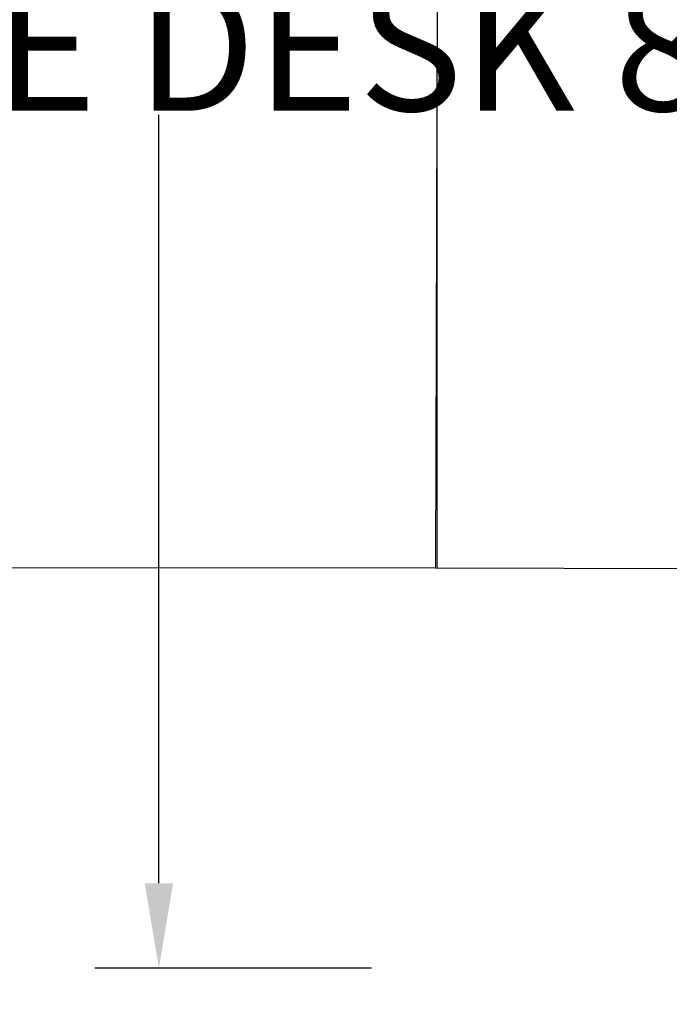
# Model space of a CAD drawing. Units: inches. Extents: x -466983 to 1020, y 324 to 318697.
# Tile 32 of 97: x 817 to 848, y 734 to 781. Entities that reach past the tile are written whole.
import ezdxf

# ---------------------------------------------------------------- set-up
doc = ezdxf.new("R2010")
doc.units = ezdxf.units.IN
doc.header["$MEASUREMENT"] = 0
for name, color, linetype, lineweight in [('A-ANNO-DIMS', 2, 'Continuous', 18), ('A-FLOR-PATT', 252, 'Continuous', 13), ('A-FURN', 8, 'Continuous', 18)]:
    doc.layers.add(name, color=color, linetype=linetype, lineweight=lineweight)
doc.layers.add('Office Desk', color=30, linetype='Continuous', true_color=0xeb7500)
doc.styles.get("Standard").update_dxf_attribs({"font": 'arial.ttf'})
doc.dimstyles.get("Standard").update_dxf_attribs({"dimtxt": 6, "dimasz": 4, "dimexe": 3, "dimexo": 3, "dimgap": 0.09, "dimtad": 0, "dimtih": 1, "dimtoh": 1, "dimdec": 1, "dimzin": 0, "dimdsep": 46, "dimlunit": 3, "dimtxsty": 'Standard', "dimcen": 0.09, "dimadec": 0, "dimazin": 0, "dimtfac": 1, "dimtdec": 1, "dimtofl": 0, "dimtmove": 0, "dimatfit": 3, "dimfxl": 1, "dimtolj": 1, "dimtzin": 0, "dimarcsym": 0})

# ---------------------------------------------------------------- blocks, each defined once
blk = doc.blocks.new('Offce Table')
at = {"layer": 'Office Desk'}
for p, q in [((2575.742, 981.616, -0.016), (2575.658, 950.355, -0.016)), ((2575.658, 950.355, -0.016), (2635.658, 950.194, -0.016))]:
    blk.add_line(p, q, dxfattribs=at)
blk = doc.blocks.new('Office Desk With Chairs')
blk.add_blockref('Offce Table', (-526.404, 94.584))
blk = doc.blocks.new('*D99')
at = {"layer": 'A-ANNO-DIMS', "color": 0, "lineweight": -2, "transparency": 16777216}
for p, q in [((833.84, 822.679), (820.85, 822.679)), ((823.85, 818.679), (823.85, 782.572)), ((823.85, 740.077), (823.85, 776.184)), ((833.84, 736.077), (820.85, 736.077))]:
    blk.add_line(p, q, dxfattribs=at)
at = {"layer": 'A-ANNO-DIMS', "color": 0, "transparency": 16777216}
for points in [[(823.183, 818.679), (824.517, 818.679), (823.85, 822.679)], [(823.183, 740.077), (824.517, 740.077), (823.85, 736.077)]]:
    blk.add_solid(points, dxfattribs=at)
at = {"layer": 'Defpoints', "color": 0, "transparency": 16777216}
for p in [(823.85, 822.679), (836.84, 822.679), (836.84, 736.077)]:
    blk.add_point(p, dxfattribs=at)
at = {"layer": 'A-ANNO-DIMS', "color": 0, "transparency": 16777216, "insert": (823.85, 779.378), "char_height": 6, "attachment_point": 5}
blk.add_mtext('\\A1;OFFICE DESK 87', dxfattribs=at)

msp = doc.modelspace()

# ---------------------------------------------------------------- hatches: boundary and pattern name
at = {"layer": 'A-FLOR-PATT', "transparency": 33554572}
h = msp.add_hatch(dxfattribs=at)
h.set_pattern_fill('ANSI37', color=256, scale=30)
h.set_pattern_definition([(45, (-1212.4137, -290.035), (-2.6516504, 2.6516504), []), (135, (-1212.4137, -290.035), (-2.6516504, -2.6516504), [])])
h.paths.add_polyline_path([(901.806, 1075.938), (900.614, 1075.938), (900.614, 1065.386), (899.391, 1065.386), (898.091, 1065.386), (892.836, 1058.71, -0.258377), (892.188, 1058.351), (879.985, 1058.351, -0.20177), (879.438, 1058.581), (874.081, 1065.386), (872.781, 1065.386), (871.558, 1065.386), (871.558, 1075.938), (813.806, 1075.938), (813.806, 1044.792), (832.395, 1044.792, -0.394795), (848.66, 1028.536), (848.66, 1009.938), (901.806, 1009.938), (901.806, 1015.938), (901.306, 1015.938), (871.306, 1015.938), (871.306, 1017.25), (871.334, 1017.25, -0.401453), (901.306, 1045.938), (901.806, 1045.938)])
edge = h.paths.add_edge_path(flags=16)
edge.add_line((847.773, 1068.949), (847.773, 1073.709))
edge.add_arc((849.227, 1073.709), 1.454, 90, 180, ccw=False)
edge.add_line((849.227, 1075.163), (864.492, 1075.163))
edge.add_arc((864.492, 1073.709), 1.454, 0, 90, ccw=False)
edge.add_line((865.946, 1073.709), (865.946, 1069.004))
edge.add_arc((832.645, 1068.976), 33.301, -20.6123, 0.0472, ccw=False)
edge.add_ellipse((856.859, 1058.48), major_axis=(0, 10.213), ratio=0.685919, start_angle=100.0088, end_angle=259.9912, ccw=False)
edge.add_arc((881.074, 1068.976), 33.301, 180.0472, 200.6123, ccw=False)
h.paths.add_polyline_path([(853.146, 1066.482), (853.146, 1066.453), (853.146, 1066.453, 0.433107), (852.917, 1066.685), (852.917, 1066.453), (853.146, 1066.453), (853.146, 1066.482), (853.088, 1066.612, 0.697939), (852.7, 1066.453), (852.7, 1066.453), (852.7, 1066.482), (852.917, 1067.001), (852.917, 1066.685, -0.396254)], flags=0)
h.paths.add_polyline_path([(861.019, 1066.482), (861.019, 1066.453), (861.019, 1066.453, 0.416404), (860.802, 1066.685), (860.802, 1066.453), (861.019, 1066.453), (861.019, 1066.482), (860.967, 1066.605, 0.713344), (860.573, 1066.453), (860.573, 1066.453), (860.573, 1066.482), (860.802, 1067.001), (860.802, 1066.685, -0.379973)], flags=0)
edge = h.paths.add_edge_path(flags=0)
edge.add_spline(control_points=[(861.13, 1065.785), (861.466, 1065.248), (861.613, 1065.016), (861.983, 1064.374), (862.192, 1063.944), (862.561, 1063.039), (862.721, 1062.563), (862.987, 1061.578), (863.092, 1061.069), (863.245, 1060.031), (863.293, 1059.503), (863.329, 1058.441), (863.318, 1057.908), (863.237, 1056.852), (863.166, 1056.329), (862.97, 1055.308), (862.843, 1054.81), (862.537, 1053.852), (862.357, 1053.393), (861.951, 1052.525), (861.725, 1052.117), (861.233, 1051.362), (860.967, 1051.016), (860.405, 1050.395), (860.108, 1050.12), (859.494, 1049.646), (859.176, 1049.448), (858.528, 1049.13), (858.197, 1049.011), (857.531, 1048.852), (857.196, 1048.812), (856.525, 1048.812), (856.189, 1048.852), (855.524, 1049.01), (855.193, 1049.129), (854.545, 1049.447), (854.227, 1049.645), (853.612, 1050.118), (853.316, 1050.393), (852.753, 1051.014), (852.487, 1051.36), (851.995, 1052.114), (851.769, 1052.523), (851.363, 1053.39), (851.183, 1053.85), (850.877, 1054.807), (850.75, 1055.305), (850.553, 1056.326), (850.483, 1056.849), (850.401, 1057.905), (850.39, 1058.438), (850.426, 1059.5), (850.473, 1060.028), (850.626, 1061.066), (850.732, 1061.575), (850.997, 1062.561), (851.157, 1063.036), (851.525, 1063.942), (851.734, 1064.371), (852.106, 1065.016), (852.254, 1065.25), (852.608, 1065.733)], knot_values=[3.915332, 3.915332, 3.915332, 3.915332, 4.013468, 4.013468, 4.175532, 4.175532, 4.337596, 4.337596, 4.49966, 4.49966, 4.661724, 4.661724, 4.823788, 4.823788, 4.985852, 4.985852, 5.147916, 5.147916, 5.30998, 5.30998, 5.472044, 5.472044, 5.634109, 5.634109, 5.796173, 5.796173, 5.958237, 5.958237, 6.120301, 6.120301, 6.282365, 6.282365, 6.444429, 6.444429, 6.606493, 6.606493, 6.768557, 6.768557, 6.930621, 6.930621, 7.092685, 7.092685, 7.254749, 7.254749, 7.416813, 7.416813, 7.578878, 7.578878, 7.740942, 7.740942, 7.903006, 7.903006, 8.06507, 8.06507, 8.227134, 8.227134, 8.389198, 8.389198, 8.551262, 8.551262, 8.65037, 8.65037, 8.65037, 8.65037], degree=3, periodic=0)
edge.add_line((852.642, 1065.785), (861.13, 1065.785))
edge = h.paths.add_edge_path(flags=0)
edge.add_ellipse((856.85, 1057.743), major_axis=(0, 7.792), ratio=0.687861, start_angle=0, end_angle=360)
h.paths.add_polyline_path([(848.863, 1069.389), (848.863, 1073.96, -0.414214), (849.954, 1075.051), (863.765, 1075.051, -0.414214), (864.856, 1073.96), (864.856, 1069.389, -0.388936), (864.524, 1069.027, -0.043561), (849.195, 1069.027, -0.388936)], flags=0)
h.paths.add_polyline_path([(853.101, 1068.112, -1), (852.677, 1068.112, -1)], flags=0)
edge = h.paths.add_edge_path(flags=0)
edge.add_ellipse((856.859, 1057.338), major_axis=(0, 2.207), ratio=0.657164, start_angle=0, end_angle=360)
h.paths.add_polyline_path([(861.041, 1068.112, -1), (860.618, 1068.112, -1)], flags=0)
edge = h.paths.add_edge_path()
edge.add_line((573.954, 1057.341), (573.954, 1075.938))
edge.add_line((573.954, 1075.938), (558.731, 1075.938))
edge.add_line((558.731, 1075.938), (558.731, 1065.386))
edge.add_line((558.731, 1065.386), (557.507, 1065.386))
edge.add_line((557.507, 1065.386), (556.207, 1065.386))
edge.add_line((556.207, 1065.386), (550.952, 1058.71))
edge.add_arc((550.304, 1059.116), 0.765, 270, 327.9483, ccw=False)
edge.add_line((550.304, 1058.351), (538.101, 1058.351))
edge.add_arc((538.101, 1059.116), 0.765, 224.3704, 270, ccw=False)
edge.add_line((537.555, 1058.581), (532.198, 1065.386))
edge.add_line((532.198, 1065.386), (530.898, 1065.386))
edge.add_line((530.898, 1065.386), (529.674, 1065.386))
edge.add_line((529.674, 1065.386), (529.674, 1075.938))
edge.add_line((529.674, 1075.938), (520.806, 1075.938))
edge.add_line((520.806, 1075.938), (520.806, 1045.938))
edge.add_line((520.806, 1045.938), (521.306, 1045.938))
edge.add_arc((521.306, 1015.938), 30, 2.5075, 90, ccw=False)
edge.add_line((551.277, 1017.25), (551.306, 1017.25))
edge.add_line((551.306, 1017.25), (551.306, 1015.938))
edge.add_line((551.306, 1015.938), (520.806, 1015.938))
edge.add_line((520.806, 1015.938), (520.806, 1009.938))
edge.add_line((520.806, 1009.938), (559.191, 1010.402))
edge.add_arc((559.191, 1011.856), 1.454, 180, 270, ccw=False)
edge.add_line((557.737, 1011.856), (557.737, 1016.561))
edge.add_arc((591.039, 1016.589), 33.301, 159.3877, 180.0472, ccw=False)
edge.add_ellipse((566.824, 1027.085), major_axis=(0, 10.213), ratio=0.685919, start_angle=280.0088, end_angle=439.9912, ccw=False)
edge.add_arc((542.609, 1016.589), 33.301, 0.0472, 20.6123, ccw=False)
edge.add_line((575.91, 1016.616), (575.91, 1011.856))
edge.add_arc((574.456, 1011.856), 1.454, -90, 0, ccw=False)
edge.add_line((574.456, 1010.402), (608.806, 1009.938))
edge.add_line((608.806, 1009.938), (608.806, 1041.086))
edge.add_line((608.806, 1041.086), (590.218, 1041.086))
edge.add_arc((590.775, 1057.907), 16.831, 181.9277, 268.1032, ccw=False)
edge = h.paths.add_edge_path()
edge.add_ellipse((494.244, 583.62), major_axis=(0, 10.213), ratio=0.685919, start_angle=280.0088, end_angle=439.9912, ccw=False)
edge.add_arc((470.03, 573.124), 33.301, 0.0472, 20.6123, ccw=False)
edge.add_line((503.331, 573.152), (503.331, 568.392))
edge.add_arc((501.877, 568.392), 1.454, -90, 0, ccw=False)
edge.add_line((501.877, 566.938), (539.806, 566.938))
edge.add_line((539.806, 566.938), (539.806, 572.938))
edge.add_line((539.806, 572.938), (539.306, 572.938))
edge.add_line((539.306, 572.938), (509.306, 572.938))
edge.add_line((509.306, 572.938), (509.306, 574.25))
edge.add_line((509.306, 574.25), (509.334, 574.25))
edge.add_arc((539.306, 572.938), 30, 90, 177.4925, ccw=False)
edge.add_line((539.306, 602.938), (539.806, 602.938))
edge.add_line((539.806, 602.938), (539.806, 626.938))
edge.add_line((539.806, 626.938), (531.772, 626.938))
edge.add_line((531.772, 626.938), (531.772, 616.386))
edge.add_line((531.772, 616.386), (530.548, 616.386))
edge.add_line((530.548, 616.386), (529.249, 616.386))
edge.add_line((529.249, 616.386), (523.711, 609.351))
edge.add_line((523.711, 609.351), (510.777, 609.351))
edge.add_line((510.777, 609.351), (505.239, 616.386))
edge.add_line((505.239, 616.386), (503.939, 616.386))
edge.add_line((503.939, 616.386), (502.715, 616.386))
edge.add_line((502.715, 616.386), (502.715, 626.938))
edge.add_line((502.715, 626.938), (481.698, 626.938))
edge.add_line((481.698, 626.938), (481.698, 610.995))
edge.add_arc((467.27, 611.473), 14.436, 271.9277, 358.1032, ccw=False)
edge.add_line((467.756, 597.045), (451.806, 597.045))
edge.add_line((451.806, 597.045), (451.806, 584.404))
edge.add_line((451.806, 584.404), (451.806, 566.938))
edge.add_line((451.806, 566.938), (486.612, 566.938))
edge.add_arc((486.612, 568.392), 1.454, 180, 270, ccw=False)
edge.add_line((485.158, 568.392), (485.158, 573.097))
edge.add_arc((518.459, 573.124), 33.301, 159.3877, 180.0472, ccw=False)
h.paths.add_polyline_path([(836.261, 1020.733), (879.89, 1020.733), (879.89, 1039.39), (836.261, 1039.39)], flags=25)
h.paths.add_polyline_path([(549.985, 1036.749), (593.614, 1036.749), (593.614, 1055.407), (549.985, 1055.407)], flags=24)
h.paths.add_polyline_path([(475.123, 595.596), (518.752, 595.596), (518.752, 614.253), (475.123, 614.253)], flags=24)

# ---------------------------------------------------------------- linework, layer by layer
at = {"layer": 'A-FURN', "elevation": -0.016}
msp.add_lwpolyline([(836.84, 754.904), (813.806, 754.904), (813.806, 824.938), (836.924, 824.938), (836.924, 754.904)], dxfattribs=at)

# ---------------------------------------------------------------- block references
at = {"layer": 'A-FURN'}
msp.add_blockref('Office Desk With Chairs', (-1212.414, -290.035), dxfattribs=at)

# ---------------------------------------------------------------- dimensions: what is measured, and where the dimension line sits
at = {"layer": 'A-ANNO-DIMS'}
dim = msp.add_linear_dim(base=(823.85, 822.679), p1=(836.84, 736.077), p2=(836.84, 822.679), angle=90, text='OFFICE DESK <>', dimstyle='Standard', override={"dimdec": 0, "dimlfac": 1, "dimrnd": 0, "dimzin": 0, "dimdsep": 46, "dimlunit": 2}, dxfattribs=at)
dim.commit()
dim.dimension.update_dxf_attribs({"geometry": '*D99', "text_midpoint": (823.85, 779.378)})

doc.saveas('drawing.dxf')
